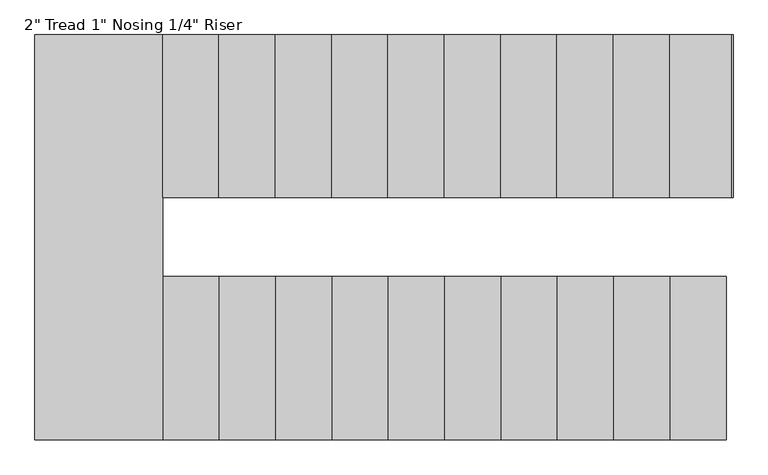
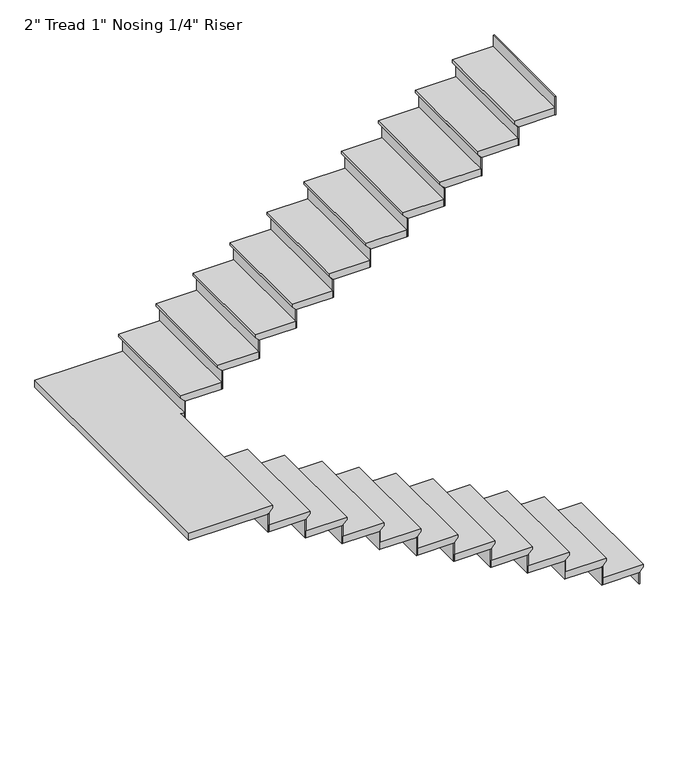
"""IFC4 building model written with IfcOpenShell, lengths in millimetres: stair flight geometry."""

from ifc_helpers import new_model, si_unit, origin, place, context, project, spatial, faceted_brep, source, transform, mapped, element, save


def stair_flight_8de044e6(model_context):
    return source(origin(), model_context, "Body", "Brep", [
        faceted_brep([(-3117.2664982, -6914.3822004, 3312.9681818), (-3117.2664982, -6914.3822004, 3332.0181818), (-3117.2664982, -7650.9822004, 3332.0181818), (-3117.2664982, -7650.9822004, 3312.9681818), (-3142.6664982, -6914.3822004, 3287.5681818), (-3142.6664982, -7650.9822004, 3287.5681818), (-3396.6664982, -6914.3822004, 3332.0181818), (-3396.6664982, -7650.9822004, 3332.0181818), (-3142.6664982, -7650.9822004, 3281.2181818), (-3396.6664982, -7650.9822004, 3281.2181818), (-3396.6664982, -6914.3822004, 3281.2181818), (-3142.6664982, -6914.3822004, 3281.2181818)], [[[0, 1, 2, 3]], [[4, 0, 3, 5]], [[2, 1, 6, 7]], [[8, 9, 10, 11]], [[2, 7, 9, 8, 5, 3]], [[8, 11, 4, 5]], [[6, 1, 0, 4, 11, 10]], [[7, 6, 10, 9]]]),
        faceted_brep([(-3142.6664982, -6914.3822004, 3281.2181818), (-3142.6664982, -6914.3822004, 3200.4), (-3149.0164982, -6914.3822004, 3200.4), (-3149.0164982, -6914.3822004, 3281.2181818), (-3142.6664982, -7650.9822004, 3281.2181818), (-3149.0164982, -7650.9822004, 3281.2181818), (-3149.0164982, -7650.9822004, 3200.4), (-3142.6664982, -7650.9822004, 3200.4)], [[[0, 1, 2, 3]], [[4, 5, 6, 7]], [[1, 0, 4, 7]], [[2, 1, 7, 6]], [[3, 2, 6, 5]], [[0, 3, 5, 4]]]),
        faceted_brep([(-3396.6664982, -6914.3822004, 3412.8363636), (-3396.6664982, -6914.3822004, 3281.2181818), (-3403.0164982, -6914.3822004, 3281.2181818), (-3403.0164982, -6914.3822004, 3412.8363636), (-3396.6664982, -7650.9822004, 3412.8363636), (-3403.0164982, -7650.9822004, 3412.8363636), (-3403.0164982, -7650.9822004, 3281.2181818), (-3396.6664982, -7650.9822004, 3281.2181818)], [[[0, 1, 2, 3]], [[4, 5, 6, 7]], [[1, 0, 4, 7]], [[2, 1, 7, 6]], [[3, 2, 6, 5]], [[0, 3, 5, 4]]]),
        faceted_brep([(-3371.2664982, -7650.9822004, 3463.6363636), (-3371.2664982, -6914.3822004, 3463.6363636), (-3650.6664982, -6914.3822004, 3463.6363636), (-3650.6664982, -7650.9822004, 3463.6363636), (-3396.6664982, -7650.9822004, 3412.8363636), (-3650.6664982, -7650.9822004, 3412.8363636), (-3650.6664982, -6914.3822004, 3412.8363636), (-3396.6664982, -6914.3822004, 3412.8363636), (-3396.6664982, -7650.9822004, 3419.1863636), (-3371.2664982, -7650.9822004, 3444.5863636), (-3396.6664982, -6914.3822004, 3419.1863636), (-3371.2664982, -6914.3822004, 3444.5863636)], [[[0, 1, 2, 3]], [[4, 5, 6, 7]], [[0, 3, 5, 4, 8, 9]], [[4, 7, 10, 8]], [[2, 1, 11, 10, 7, 6]], [[3, 2, 6, 5]], [[11, 1, 0, 9]], [[10, 11, 9, 8]]]),
        faceted_brep([(-3650.6664982, -6914.3822004, 3544.4545455), (-3650.6664982, -6914.3822004, 3412.8363636), (-3657.0164982, -6914.3822004, 3412.8363636), (-3657.0164982, -6914.3822004, 3544.4545455), (-3650.6664982, -7650.9822004, 3544.4545455), (-3657.0164982, -7650.9822004, 3544.4545455), (-3657.0164982, -7650.9822004, 3412.8363636), (-3650.6664982, -7650.9822004, 3412.8363636)], [[[0, 1, 2, 3]], [[4, 5, 6, 7]], [[1, 0, 4, 7]], [[2, 1, 7, 6]], [[3, 2, 6, 5]], [[0, 3, 5, 4]]]),
        faceted_brep([(-3625.2664982, -7650.9822004, 3595.2545455), (-3625.2664982, -6914.3822004, 3595.2545455), (-3904.6664982, -6914.3822004, 3595.2545455), (-3904.6664982, -7650.9822004, 3595.2545455), (-3650.6664982, -7650.9822004, 3544.4545455), (-3904.6664982, -7650.9822004, 3544.4545455), (-3904.6664982, -6914.3822004, 3544.4545455), (-3650.6664982, -6914.3822004, 3544.4545455), (-3650.6664982, -7650.9822004, 3550.8045455), (-3625.2664982, -7650.9822004, 3576.2045455), (-3650.6664982, -6914.3822004, 3550.8045455), (-3625.2664982, -6914.3822004, 3576.2045455)], [[[0, 1, 2, 3]], [[4, 5, 6, 7]], [[0, 3, 5, 4, 8, 9]], [[4, 7, 10, 8]], [[2, 1, 11, 10, 7, 6]], [[3, 2, 6, 5]], [[11, 1, 0, 9]], [[10, 11, 9, 8]]]),
        faceted_brep([(-3904.6664982, -6914.3822004, 3676.0727273), (-3904.6664982, -6914.3822004, 3544.4545455), (-3911.0164982, -6914.3822004, 3544.4545455), (-3911.0164982, -6914.3822004, 3676.0727273), (-3904.6664982, -7650.9822004, 3676.0727273), (-3911.0164982, -7650.9822004, 3676.0727273), (-3911.0164982, -7650.9822004, 3544.4545455), (-3904.6664982, -7650.9822004, 3544.4545455)], [[[0, 1, 2, 3]], [[4, 5, 6, 7]], [[1, 0, 4, 7]], [[2, 1, 7, 6]], [[3, 2, 6, 5]], [[0, 3, 5, 4]]]),
        faceted_brep([(-3879.2664982, -7650.9822004, 3726.8727273), (-3879.2664982, -6914.3822004, 3726.8727273), (-4158.6664982, -6914.3822004, 3726.8727273), (-4158.6664982, -7650.9822004, 3726.8727273), (-3904.6664982, -7650.9822004, 3676.0727273), (-4158.6664982, -7650.9822004, 3676.0727273), (-4158.6664982, -6914.3822004, 3676.0727273), (-3904.6664982, -6914.3822004, 3676.0727273), (-3904.6664982, -7650.9822004, 3682.4227273), (-3879.2664982, -7650.9822004, 3707.8227273), (-3904.6664982, -6914.3822004, 3682.4227273), (-3879.2664982, -6914.3822004, 3707.8227273)], [[[0, 1, 2, 3]], [[4, 5, 6, 7]], [[0, 3, 5, 4, 8, 9]], [[4, 7, 10, 8]], [[2, 1, 11, 10, 7, 6]], [[3, 2, 6, 5]], [[11, 1, 0, 9]], [[10, 11, 9, 8]]]),
        faceted_brep([(-4158.6664982, -6914.3822004, 3807.6909091), (-4158.6664982, -6914.3822004, 3676.0727273), (-4165.0164982, -6914.3822004, 3676.0727273), (-4165.0164982, -6914.3822004, 3807.6909091), (-4158.6664982, -7650.9822004, 3807.6909091), (-4165.0164982, -7650.9822004, 3807.6909091), (-4165.0164982, -7650.9822004, 3676.0727273), (-4158.6664982, -7650.9822004, 3676.0727273)], [[[0, 1, 2, 3]], [[4, 5, 6, 7]], [[1, 0, 4, 7]], [[2, 1, 7, 6]], [[3, 2, 6, 5]], [[0, 3, 5, 4]]]),
        faceted_brep([(-4133.2664982, -7650.9822004, 3858.4909091), (-4133.2664982, -6914.3822004, 3858.4909091), (-4412.6664982, -6914.3822004, 3858.4909091), (-4412.6664982, -7650.9822004, 3858.4909091), (-4158.6664982, -7650.9822004, 3807.6909091), (-4412.6664982, -7650.9822004, 3807.6909091), (-4412.6664982, -6914.3822004, 3807.6909091), (-4158.6664982, -6914.3822004, 3807.6909091), (-4158.6664982, -7650.9822004, 3814.0409091), (-4133.2664982, -7650.9822004, 3839.4409091), (-4158.6664982, -6914.3822004, 3814.0409091), (-4133.2664982, -6914.3822004, 3839.4409091)], [[[0, 1, 2, 3]], [[4, 5, 6, 7]], [[0, 3, 5, 4, 8, 9]], [[4, 7, 10, 8]], [[2, 1, 11, 10, 7, 6]], [[3, 2, 6, 5]], [[11, 1, 0, 9]], [[10, 11, 9, 8]]]),
        faceted_brep([(-4412.6664982, -6914.3822004, 3939.3090909), (-4412.6664982, -6914.3822004, 3807.6909091), (-4419.0164982, -6914.3822004, 3807.6909091), (-4419.0164982, -6914.3822004, 3939.3090909), (-4412.6664982, -7650.9822004, 3939.3090909), (-4419.0164982, -7650.9822004, 3939.3090909), (-4419.0164982, -7650.9822004, 3807.6909091), (-4412.6664982, -7650.9822004, 3807.6909091)], [[[0, 1, 2, 3]], [[4, 5, 6, 7]], [[1, 0, 4, 7]], [[2, 1, 7, 6]], [[3, 2, 6, 5]], [[0, 3, 5, 4]]]),
        faceted_brep([(-4387.2664982, -7650.9822004, 3990.1090909), (-4387.2664982, -6914.3822004, 3990.1090909), (-4666.6664982, -6914.3822004, 3990.1090909), (-4666.6664982, -7650.9822004, 3990.1090909), (-4412.6664982, -7650.9822004, 3939.3090909), (-4666.6664982, -7650.9822004, 3939.3090909), (-4666.6664982, -6914.3822004, 3939.3090909), (-4412.6664982, -6914.3822004, 3939.3090909), (-4412.6664982, -7650.9822004, 3945.6590909), (-4387.2664982, -7650.9822004, 3971.0590909), (-4412.6664982, -6914.3822004, 3945.6590909), (-4387.2664982, -6914.3822004, 3971.0590909)], [[[0, 1, 2, 3]], [[4, 5, 6, 7]], [[0, 3, 5, 4, 8, 9]], [[4, 7, 10, 8]], [[2, 1, 11, 10, 7, 6]], [[3, 2, 6, 5]], [[11, 1, 0, 9]], [[10, 11, 9, 8]]]),
        faceted_brep([(-4666.6664982, -6914.3822004, 4070.9272727), (-4666.6664982, -6914.3822004, 3939.3090909), (-4673.0164982, -6914.3822004, 3939.3090909), (-4673.0164982, -6914.3822004, 4070.9272727), (-4666.6664982, -7650.9822004, 4070.9272727), (-4673.0164982, -7650.9822004, 4070.9272727), (-4673.0164982, -7650.9822004, 3939.3090909), (-4666.6664982, -7650.9822004, 3939.3090909)], [[[0, 1, 2, 3]], [[4, 5, 6, 7]], [[1, 0, 4, 7]], [[2, 1, 7, 6]], [[3, 2, 6, 5]], [[0, 3, 5, 4]]]),
        faceted_brep([(-4641.2664982, -7650.9822004, 4121.7272727), (-4641.2664982, -6914.3822004, 4121.7272727), (-4920.6664982, -6914.3822004, 4121.7272727), (-4920.6664982, -7650.9822004, 4121.7272727), (-4666.6664982, -7650.9822004, 4070.9272727), (-4920.6664982, -7650.9822004, 4070.9272727), (-4920.6664982, -6914.3822004, 4070.9272727), (-4666.6664982, -6914.3822004, 4070.9272727), (-4666.6664982, -7650.9822004, 4077.2772727), (-4641.2664982, -7650.9822004, 4102.6772727), (-4666.6664982, -6914.3822004, 4077.2772727), (-4641.2664982, -6914.3822004, 4102.6772727)], [[[0, 1, 2, 3]], [[4, 5, 6, 7]], [[0, 3, 5, 4, 8, 9]], [[4, 7, 10, 8]], [[2, 1, 11, 10, 7, 6]], [[3, 2, 6, 5]], [[11, 1, 0, 9]], [[10, 11, 9, 8]]]),
        faceted_brep([(-4920.6664982, -6914.3822004, 4202.5454545), (-4920.6664982, -6914.3822004, 4070.9272727), (-4927.0164982, -6914.3822004, 4070.9272727), (-4927.0164982, -6914.3822004, 4202.5454545), (-4920.6664982, -7650.9822004, 4202.5454545), (-4927.0164982, -7650.9822004, 4202.5454545), (-4927.0164982, -7650.9822004, 4070.9272727), (-4920.6664982, -7650.9822004, 4070.9272727)], [[[0, 1, 2, 3]], [[4, 5, 6, 7]], [[1, 0, 4, 7]], [[2, 1, 7, 6]], [[3, 2, 6, 5]], [[0, 3, 5, 4]]]),
        faceted_brep([(-4895.2664982, -7650.9822004, 4253.3454545), (-4895.2664982, -6914.3822004, 4253.3454545), (-5174.6664982, -6914.3822004, 4253.3454545), (-5174.6664982, -7650.9822004, 4253.3454545), (-4920.6664982, -7650.9822004, 4202.5454545), (-5174.6664982, -7650.9822004, 4202.5454545), (-5174.6664982, -6914.3822004, 4202.5454545), (-4920.6664982, -6914.3822004, 4202.5454545), (-4920.6664982, -7650.9822004, 4208.8954545), (-4895.2664982, -7650.9822004, 4234.2954545), (-4920.6664982, -6914.3822004, 4208.8954545), (-4895.2664982, -6914.3822004, 4234.2954545)], [[[0, 1, 2, 3]], [[4, 5, 6, 7]], [[0, 3, 5, 4, 8, 9]], [[4, 7, 10, 8]], [[2, 1, 11, 10, 7, 6]], [[3, 2, 6, 5]], [[11, 1, 0, 9]], [[10, 11, 9, 8]]]),
        faceted_brep([(-5174.6664982, -6914.3822004, 4334.1636364), (-5174.6664982, -6914.3822004, 4202.5454545), (-5181.0164982, -6914.3822004, 4202.5454545), (-5181.0164982, -6914.3822004, 4334.1636364), (-5174.6664982, -7650.9822004, 4334.1636364), (-5181.0164982, -7650.9822004, 4334.1636364), (-5181.0164982, -7650.9822004, 4202.5454545), (-5174.6664982, -7650.9822004, 4202.5454545)], [[[0, 1, 2, 3]], [[4, 5, 6, 7]], [[1, 0, 4, 7]], [[2, 1, 7, 6]], [[3, 2, 6, 5]], [[0, 3, 5, 4]]]),
        faceted_brep([(-5149.2664982, -7650.9822004, 4384.9636364), (-5149.2664982, -6914.3822004, 4384.9636364), (-5428.6664982, -6914.3822004, 4384.9636364), (-5428.6664982, -7650.9822004, 4384.9636364), (-5174.6664982, -7650.9822004, 4334.1636364), (-5428.6664982, -7650.9822004, 4334.1636364), (-5428.6664982, -6914.3822004, 4334.1636364), (-5174.6664982, -6914.3822004, 4334.1636364), (-5174.6664982, -7650.9822004, 4340.5136364), (-5149.2664982, -7650.9822004, 4365.9136364), (-5174.6664982, -6914.3822004, 4340.5136364), (-5149.2664982, -6914.3822004, 4365.9136364)], [[[0, 1, 2, 3]], [[4, 5, 6, 7]], [[0, 3, 5, 4, 8, 9]], [[4, 7, 10, 8]], [[2, 1, 11, 10, 7, 6]], [[3, 2, 6, 5]], [[11, 1, 0, 9]], [[10, 11, 9, 8]]]),
        faceted_brep([(-5428.6664982, -6914.3822004, 4465.7818182), (-5428.6664982, -6914.3822004, 4334.1636364), (-5435.0164982, -6914.3822004, 4334.1636364), (-5435.0164982, -6914.3822004, 4465.7818182), (-5428.6664982, -7650.9822004, 4465.7818182), (-5435.0164982, -7650.9822004, 4465.7818182), (-5435.0164982, -7650.9822004, 4334.1636364), (-5428.6664982, -7650.9822004, 4334.1636364)], [[[0, 1, 2, 3]], [[4, 5, 6, 7]], [[1, 0, 4, 7]], [[2, 1, 7, 6]], [[3, 2, 6, 5]], [[0, 3, 5, 4]]]),
        faceted_brep([(-5403.2664982, -7650.9822004, 4516.5818182), (-5403.2664982, -6914.3822004, 4516.5818182), (-5682.6664982, -6914.3822004, 4516.5818182), (-5682.6664982, -7650.9822004, 4516.5818182), (-5428.6664982, -7650.9822004, 4465.7818182), (-5682.6664982, -7650.9822004, 4465.7818182), (-5682.6664982, -6914.3822004, 4465.7818182), (-5428.6664982, -6914.3822004, 4465.7818182), (-5428.6664982, -7650.9822004, 4472.1318182), (-5403.2664982, -7650.9822004, 4497.5318182), (-5428.6664982, -6914.3822004, 4472.1318182), (-5403.2664982, -6914.3822004, 4497.5318182)], [[[0, 1, 2, 3]], [[4, 5, 6, 7]], [[0, 3, 5, 4, 8, 9]], [[4, 7, 10, 8]], [[2, 1, 11, 10, 7, 6]], [[3, 2, 6, 5]], [[11, 1, 0, 9]], [[10, 11, 9, 8]]]),
        faceted_brep([(-5682.6664982, -6914.3822004, 4597.4), (-5682.6664982, -6914.3822004, 4465.7818182), (-5689.0164982, -6914.3822004, 4465.7818182), (-5689.0164982, -6914.3822004, 4597.4), (-5682.6664982, -7650.9822004, 4597.4), (-5689.0164982, -7650.9822004, 4597.4), (-5689.0164982, -7650.9822004, 4465.7818182), (-5682.6664982, -7650.9822004, 4465.7818182)], [[[0, 1, 2, 3]], [[4, 5, 6, 7]], [[1, 0, 4, 7]], [[2, 1, 7, 6]], [[3, 2, 6, 5]], [[0, 3, 5, 4]]]),
        faceted_brep([(-5631.8664982, -5824.7082131, 4648.2), (-6232.5131972, -5824.7082131, 4648.2), (-6232.5131972, -7650.9822004, 4648.2), (-5657.2664982, -7650.9822004, 4648.2), (-5657.2664982, -6558.7822004, 4648.2), (-5631.8664982, -6558.7822004, 4648.2), (-6232.5131972, -5824.7082131, 4597.4), (-5631.8664982, -5824.7082131, 4597.4), (-5631.8664982, -6558.7822004, 4597.4), (-5657.2664982, -6558.7822004, 4597.4), (-5657.2664982, -6914.3822004, 4597.4), (-5682.6664982, -6914.3822004, 4597.4), (-5682.6664982, -7650.9822004, 4597.4), (-6232.5131972, -7650.9822004, 4597.4), (-5682.6664982, -6914.3822004, 4603.75), (-5682.6664982, -7650.9822004, 4603.75), (-5657.2664982, -7650.9822004, 4629.15), (-5657.2664982, -6914.3822004, 4629.15)], [[[0, 1, 2, 3, 4, 5]], [[6, 7, 8, 9, 10, 11, 12, 13]], [[1, 0, 7, 6]], [[2, 1, 6, 13]], [[12, 11, 14, 15]], [[4, 3, 16, 17, 10, 9]], [[5, 4, 9, 8]], [[0, 5, 8, 7]], [[16, 15, 14, 17]], [[3, 2, 13, 12, 15, 16]], [[11, 10, 17, 14]]]),
        faceted_brep([(-5631.8664982, -6558.7822004, 4729.0181818), (-5631.8664982, -6558.7822004, 4597.4), (-5625.5164982, -6558.7822004, 4597.4), (-5625.5164982, -6558.7822004, 4729.0181818), (-5631.8664982, -5824.7082131, 4729.0181818), (-5625.5164982, -5824.7082131, 4729.0181818), (-5625.5164982, -5824.7082131, 4597.4), (-5631.8664982, -5824.7082131, 4597.4)], [[[0, 1, 2, 3]], [[4, 5, 6, 7]], [[1, 0, 4, 7]], [[2, 1, 7, 6]], [[3, 2, 6, 5]], [[0, 3, 5, 4]]]),
        faceted_brep([(-5657.2664982, -5824.7082131, 4779.8181818), (-5657.2664982, -6558.7822004, 4779.8181818), (-5377.8664982, -6558.7822004, 4779.8181818), (-5377.8664982, -5824.7082131, 4779.8181818), (-5631.8664982, -5824.7082131, 4729.0181818), (-5377.8664982, -5824.7082131, 4729.0181818), (-5377.8664982, -6558.7822004, 4729.0181818), (-5631.8664982, -6558.7822004, 4729.0181818), (-5631.8664982, -5824.7082131, 4735.3681818), (-5657.2664982, -5824.7082131, 4760.7681818), (-5631.8664982, -6558.7822004, 4735.3681818), (-5657.2664982, -6558.7822004, 4760.7681818)], [[[0, 1, 2, 3]], [[4, 5, 6, 7]], [[0, 3, 5, 4, 8, 9]], [[4, 7, 10, 8]], [[2, 1, 11, 10, 7, 6]], [[3, 2, 6, 5]], [[11, 1, 0, 9]], [[10, 11, 9, 8]]]),
        faceted_brep([(-5377.8664982, -6558.7822004, 4860.6363636), (-5377.8664982, -6558.7822004, 4729.0181818), (-5371.5164982, -6558.7822004, 4729.0181818), (-5371.5164982, -6558.7822004, 4860.6363636), (-5377.8664982, -5824.7082131, 4860.6363636), (-5371.5164982, -5824.7082131, 4860.6363636), (-5371.5164982, -5824.7082131, 4729.0181818), (-5377.8664982, -5824.7082131, 4729.0181818)], [[[0, 1, 2, 3]], [[4, 5, 6, 7]], [[1, 0, 4, 7]], [[2, 1, 7, 6]], [[3, 2, 6, 5]], [[0, 3, 5, 4]]]),
        faceted_brep([(-5403.2664982, -5824.7082131, 4911.4363636), (-5403.2664982, -6558.7822004, 4911.4363636), (-5123.8664982, -6558.7822004, 4911.4363636), (-5123.8664982, -5824.7082131, 4911.4363636), (-5377.8664982, -5824.7082131, 4860.6363636), (-5123.8664982, -5824.7082131, 4860.6363636), (-5123.8664982, -6558.7822004, 4860.6363636), (-5377.8664982, -6558.7822004, 4860.6363636), (-5377.8664982, -5824.7082131, 4866.9863636), (-5403.2664982, -5824.7082131, 4892.3863636), (-5377.8664982, -6558.7822004, 4866.9863636), (-5403.2664982, -6558.7822004, 4892.3863636)], [[[0, 1, 2, 3]], [[4, 5, 6, 7]], [[0, 3, 5, 4, 8, 9]], [[4, 7, 10, 8]], [[2, 1, 11, 10, 7, 6]], [[3, 2, 6, 5]], [[11, 1, 0, 9]], [[10, 11, 9, 8]]]),
        faceted_brep([(-5123.8664982, -6558.7822004, 4992.2545455), (-5123.8664982, -6558.7822004, 4860.6363636), (-5117.5164982, -6558.7822004, 4860.6363636), (-5117.5164982, -6558.7822004, 4992.2545455), (-5123.8664982, -5824.7082131, 4992.2545455), (-5117.5164982, -5824.7082131, 4992.2545455), (-5117.5164982, -5824.7082131, 4860.6363636), (-5123.8664982, -5824.7082131, 4860.6363636)], [[[0, 1, 2, 3]], [[4, 5, 6, 7]], [[1, 0, 4, 7]], [[2, 1, 7, 6]], [[3, 2, 6, 5]], [[0, 3, 5, 4]]]),
        faceted_brep([(-5149.2664982, -5824.7082131, 5043.0545455), (-5149.2664982, -6558.7822004, 5043.0545455), (-4869.8664982, -6558.7822004, 5043.0545455), (-4869.8664982, -5824.7082131, 5043.0545455), (-5123.8664982, -5824.7082131, 4992.2545455), (-4869.8664982, -5824.7082131, 4992.2545455), (-4869.8664982, -6558.7822004, 4992.2545455), (-5123.8664982, -6558.7822004, 4992.2545455), (-5123.8664982, -5824.7082131, 4998.6045455), (-5149.2664982, -5824.7082131, 5024.0045455), (-5123.8664982, -6558.7822004, 4998.6045455), (-5149.2664982, -6558.7822004, 5024.0045455)], [[[0, 1, 2, 3]], [[4, 5, 6, 7]], [[0, 3, 5, 4, 8, 9]], [[4, 7, 10, 8]], [[2, 1, 11, 10, 7, 6]], [[3, 2, 6, 5]], [[11, 1, 0, 9]], [[10, 11, 9, 8]]]),
        faceted_brep([(-4869.8664982, -6558.7822004, 5123.8727273), (-4869.8664982, -6558.7822004, 4992.2545455), (-4863.5164982, -6558.7822004, 4992.2545455), (-4863.5164982, -6558.7822004, 5123.8727273), (-4869.8664982, -5824.7082131, 5123.8727273), (-4863.5164982, -5824.7082131, 5123.8727273), (-4863.5164982, -5824.7082131, 4992.2545455), (-4869.8664982, -5824.7082131, 4992.2545455)], [[[0, 1, 2, 3]], [[4, 5, 6, 7]], [[1, 0, 4, 7]], [[2, 1, 7, 6]], [[3, 2, 6, 5]], [[0, 3, 5, 4]]]),
        faceted_brep([(-4895.2664982, -5824.7082131, 5174.6727273), (-4895.2664982, -6558.7822004, 5174.6727273), (-4615.8664982, -6558.7822004, 5174.6727273), (-4615.8664982, -5824.7082131, 5174.6727273), (-4869.8664982, -5824.7082131, 5123.8727273), (-4615.8664982, -5824.7082131, 5123.8727273), (-4615.8664982, -6558.7822004, 5123.8727273), (-4869.8664982, -6558.7822004, 5123.8727273), (-4869.8664982, -5824.7082131, 5130.2227273), (-4895.2664982, -5824.7082131, 5155.6227273), (-4869.8664982, -6558.7822004, 5130.2227273), (-4895.2664982, -6558.7822004, 5155.6227273)], [[[0, 1, 2, 3]], [[4, 5, 6, 7]], [[0, 3, 5, 4, 8, 9]], [[4, 7, 10, 8]], [[2, 1, 11, 10, 7, 6]], [[3, 2, 6, 5]], [[11, 1, 0, 9]], [[10, 11, 9, 8]]]),
        faceted_brep([(-4615.8664982, -6558.7822004, 5255.4909091), (-4615.8664982, -6558.7822004, 5123.8727273), (-4609.5164982, -6558.7822004, 5123.8727273), (-4609.5164982, -6558.7822004, 5255.4909091), (-4615.8664982, -5824.7082131, 5255.4909091), (-4609.5164982, -5824.7082131, 5255.4909091), (-4609.5164982, -5824.7082131, 5123.8727273), (-4615.8664982, -5824.7082131, 5123.8727273)], [[[0, 1, 2, 3]], [[4, 5, 6, 7]], [[1, 0, 4, 7]], [[2, 1, 7, 6]], [[3, 2, 6, 5]], [[0, 3, 5, 4]]]),
        faceted_brep([(-4641.2664982, -5824.7082131, 5306.2909091), (-4641.2664982, -6558.7822004, 5306.2909091), (-4361.8664982, -6558.7822004, 5306.2909091), (-4361.8664982, -5824.7082131, 5306.2909091), (-4615.8664982, -5824.7082131, 5255.4909091), (-4361.8664982, -5824.7082131, 5255.4909091), (-4361.8664982, -6558.7822004, 5255.4909091), (-4615.8664982, -6558.7822004, 5255.4909091), (-4615.8664982, -5824.7082131, 5261.8409091), (-4641.2664982, -5824.7082131, 5287.2409091), (-4615.8664982, -6558.7822004, 5261.8409091), (-4641.2664982, -6558.7822004, 5287.2409091)], [[[0, 1, 2, 3]], [[4, 5, 6, 7]], [[0, 3, 5, 4, 8, 9]], [[4, 7, 10, 8]], [[2, 1, 11, 10, 7, 6]], [[3, 2, 6, 5]], [[11, 1, 0, 9]], [[10, 11, 9, 8]]]),
        faceted_brep([(-4361.8664982, -6558.7822004, 5387.1090909), (-4361.8664982, -6558.7822004, 5255.4909091), (-4355.5164982, -6558.7822004, 5255.4909091), (-4355.5164982, -6558.7822004, 5387.1090909), (-4361.8664982, -5824.7082131, 5387.1090909), (-4355.5164982, -5824.7082131, 5387.1090909), (-4355.5164982, -5824.7082131, 5255.4909091), (-4361.8664982, -5824.7082131, 5255.4909091)], [[[0, 1, 2, 3]], [[4, 5, 6, 7]], [[1, 0, 4, 7]], [[2, 1, 7, 6]], [[3, 2, 6, 5]], [[0, 3, 5, 4]]]),
        faceted_brep([(-4387.2664982, -5824.7082131, 5437.9090909), (-4387.2664982, -6558.7822004, 5437.9090909), (-4107.8664982, -6558.7822004, 5437.9090909), (-4107.8664982, -5824.7082131, 5437.9090909), (-4361.8664982, -5824.7082131, 5387.1090909), (-4107.8664982, -5824.7082131, 5387.1090909), (-4107.8664982, -6558.7822004, 5387.1090909), (-4361.8664982, -6558.7822004, 5387.1090909), (-4361.8664982, -5824.7082131, 5393.4590909), (-4387.2664982, -5824.7082131, 5418.8590909), (-4361.8664982, -6558.7822004, 5393.4590909), (-4387.2664982, -6558.7822004, 5418.8590909)], [[[0, 1, 2, 3]], [[4, 5, 6, 7]], [[0, 3, 5, 4, 8, 9]], [[4, 7, 10, 8]], [[2, 1, 11, 10, 7, 6]], [[3, 2, 6, 5]], [[11, 1, 0, 9]], [[10, 11, 9, 8]]]),
        faceted_brep([(-4107.8664982, -6558.7822004, 5518.7272727), (-4107.8664982, -6558.7822004, 5387.1090909), (-4101.5164982, -6558.7822004, 5387.1090909), (-4101.5164982, -6558.7822004, 5518.7272727), (-4107.8664982, -5824.7082131, 5518.7272727), (-4101.5164982, -5824.7082131, 5518.7272727), (-4101.5164982, -5824.7082131, 5387.1090909), (-4107.8664982, -5824.7082131, 5387.1090909)], [[[0, 1, 2, 3]], [[4, 5, 6, 7]], [[1, 0, 4, 7]], [[2, 1, 7, 6]], [[3, 2, 6, 5]], [[0, 3, 5, 4]]]),
        faceted_brep([(-4133.2664982, -5824.7082131, 5569.5272727), (-4133.2664982, -6558.7822004, 5569.5272727), (-3853.8664982, -6558.7822004, 5569.5272727), (-3853.8664982, -5824.7082131, 5569.5272727), (-4107.8664982, -5824.7082131, 5518.7272727), (-3853.8664982, -5824.7082131, 5518.7272727), (-3853.8664982, -6558.7822004, 5518.7272727), (-4107.8664982, -6558.7822004, 5518.7272727), (-4107.8664982, -5824.7082131, 5525.0772727), (-4133.2664982, -5824.7082131, 5550.4772727), (-4107.8664982, -6558.7822004, 5525.0772727), (-4133.2664982, -6558.7822004, 5550.4772727)], [[[0, 1, 2, 3]], [[4, 5, 6, 7]], [[0, 3, 5, 4, 8, 9]], [[4, 7, 10, 8]], [[2, 1, 11, 10, 7, 6]], [[3, 2, 6, 5]], [[11, 1, 0, 9]], [[10, 11, 9, 8]]]),
        faceted_brep([(-3853.8664982, -6558.7822004, 5650.3454545), (-3853.8664982, -6558.7822004, 5518.7272727), (-3847.5164982, -6558.7822004, 5518.7272727), (-3847.5164982, -6558.7822004, 5650.3454545), (-3853.8664982, -5824.7082131, 5650.3454545), (-3847.5164982, -5824.7082131, 5650.3454545), (-3847.5164982, -5824.7082131, 5518.7272727), (-3853.8664982, -5824.7082131, 5518.7272727)], [[[0, 1, 2, 3]], [[4, 5, 6, 7]], [[1, 0, 4, 7]], [[2, 1, 7, 6]], [[3, 2, 6, 5]], [[0, 3, 5, 4]]]),
        faceted_brep([(-3879.2664982, -5824.7082131, 5701.1454545), (-3879.2664982, -6558.7822004, 5701.1454545), (-3599.8664982, -6558.7822004, 5701.1454545), (-3599.8664982, -5824.7082131, 5701.1454545), (-3853.8664982, -5824.7082131, 5650.3454545), (-3599.8664982, -5824.7082131, 5650.3454545), (-3599.8664982, -6558.7822004, 5650.3454545), (-3853.8664982, -6558.7822004, 5650.3454545), (-3853.8664982, -5824.7082131, 5656.6954545), (-3879.2664982, -5824.7082131, 5682.0954545), (-3853.8664982, -6558.7822004, 5656.6954545), (-3879.2664982, -6558.7822004, 5682.0954545)], [[[0, 1, 2, 3]], [[4, 5, 6, 7]], [[0, 3, 5, 4, 8, 9]], [[4, 7, 10, 8]], [[2, 1, 11, 10, 7, 6]], [[3, 2, 6, 5]], [[11, 1, 0, 9]], [[10, 11, 9, 8]]]),
        faceted_brep([(-3599.8664982, -6558.7822004, 5781.9636364), (-3599.8664982, -6558.7822004, 5650.3454545), (-3593.5164982, -6558.7822004, 5650.3454545), (-3593.5164982, -6558.7822004, 5781.9636364), (-3599.8664982, -5824.7082131, 5781.9636364), (-3593.5164982, -5824.7082131, 5781.9636364), (-3593.5164982, -5824.7082131, 5650.3454545), (-3599.8664982, -5824.7082131, 5650.3454545)], [[[0, 1, 2, 3]], [[4, 5, 6, 7]], [[1, 0, 4, 7]], [[2, 1, 7, 6]], [[3, 2, 6, 5]], [[0, 3, 5, 4]]]),
        faceted_brep([(-3625.2664982, -5824.7082131, 5832.7636364), (-3625.2664982, -6558.7822004, 5832.7636364), (-3345.8664982, -6558.7822004, 5832.7636364), (-3345.8664982, -5824.7082131, 5832.7636364), (-3599.8664982, -5824.7082131, 5781.9636364), (-3345.8664982, -5824.7082131, 5781.9636364), (-3345.8664982, -6558.7822004, 5781.9636364), (-3599.8664982, -6558.7822004, 5781.9636364), (-3599.8664982, -5824.7082131, 5788.3136364), (-3625.2664982, -5824.7082131, 5813.7136364), (-3599.8664982, -6558.7822004, 5788.3136364), (-3625.2664982, -6558.7822004, 5813.7136364)], [[[0, 1, 2, 3]], [[4, 5, 6, 7]], [[0, 3, 5, 4, 8, 9]], [[4, 7, 10, 8]], [[2, 1, 11, 10, 7, 6]], [[3, 2, 6, 5]], [[11, 1, 0, 9]], [[10, 11, 9, 8]]]),
        faceted_brep([(-3345.8664982, -6558.7822004, 5913.5818182), (-3345.8664982, -6558.7822004, 5781.9636364), (-3339.5164982, -6558.7822004, 5781.9636364), (-3339.5164982, -6558.7822004, 5913.5818182), (-3345.8664982, -5824.7082131, 5913.5818182), (-3339.5164982, -5824.7082131, 5913.5818182), (-3339.5164982, -5824.7082131, 5781.9636364), (-3345.8664982, -5824.7082131, 5781.9636364)], [[[0, 1, 2, 3]], [[4, 5, 6, 7]], [[1, 0, 4, 7]], [[2, 1, 7, 6]], [[3, 2, 6, 5]], [[0, 3, 5, 4]]]),
        faceted_brep([(-3091.8664982, -6558.7822004, 6045.2), (-3091.8664982, -6558.7822004, 5913.5818182), (-3085.5164982, -6558.7822004, 5913.5818182), (-3085.5164982, -6558.7822004, 6045.2), (-3091.8664982, -5824.7082131, 6045.2), (-3085.5164982, -5824.7082131, 6045.2), (-3085.5164982, -5824.7082131, 5913.5818182), (-3091.8664982, -5824.7082131, 5913.5818182)], [[[0, 1, 2, 3]], [[4, 5, 6, 7]], [[1, 0, 4, 7]], [[2, 1, 7, 6]], [[3, 2, 6, 5]], [[0, 3, 5, 4]]]),
        faceted_brep([(-3371.2664982, -5824.7082131, 5964.3818182), (-3371.2664982, -6558.7822004, 5964.3818182), (-3091.8664982, -6558.7822004, 5964.3818182), (-3091.8664982, -5824.7082131, 5964.3818182), (-3345.8664982, -5824.7082131, 5913.5818182), (-3091.8664982, -5824.7082131, 5913.5818182), (-3091.8664982, -6558.7822004, 5913.5818182), (-3345.8664982, -6558.7822004, 5913.5818182), (-3345.8664982, -5824.7082131, 5919.9318182), (-3371.2664982, -5824.7082131, 5945.3318182), (-3345.8664982, -6558.7822004, 5919.9318182), (-3371.2664982, -6558.7822004, 5945.3318182)], [[[0, 1, 2, 3]], [[4, 5, 6, 7]], [[0, 3, 5, 4, 8, 9]], [[4, 7, 10, 8]], [[2, 1, 11, 10, 7, 6]], [[3, 2, 6, 5]], [[11, 1, 0, 9]], [[10, 11, 9, 8]]]),
    ])


if __name__ == "__main__":
    model = new_model("IFC4")
    model_context = context("Model", 3, world=origin())
    ifc_project = project(units=[si_unit("LENGTHUNIT", "METRE", prefix="MILLI")], contexts=[model_context])
    site = spatial("IfcSite", under=ifc_project)
    building = spatial("IfcBuilding", under=site)
    placement = place(None, origin())
    stair_flight_shape = stair_flight_8de044e6(model_context)
    element("IfcStairFlight", 1, ObjectType="2\" Tread 1\" Nosing 1/4\" Riser", at=placement, inside=building, context=model_context, shape_type="MappedRepresentation", body=[
        mapped(stair_flight_shape, transform((0.0, 0.0, 0.0), x_axis=(1.0, 0.0, 0.0), y_axis=(0.0, 1.0, 0.0), z_axis=(0.0, 0.0, 1.0))),
    ])
    save(model, "model.ifc")
